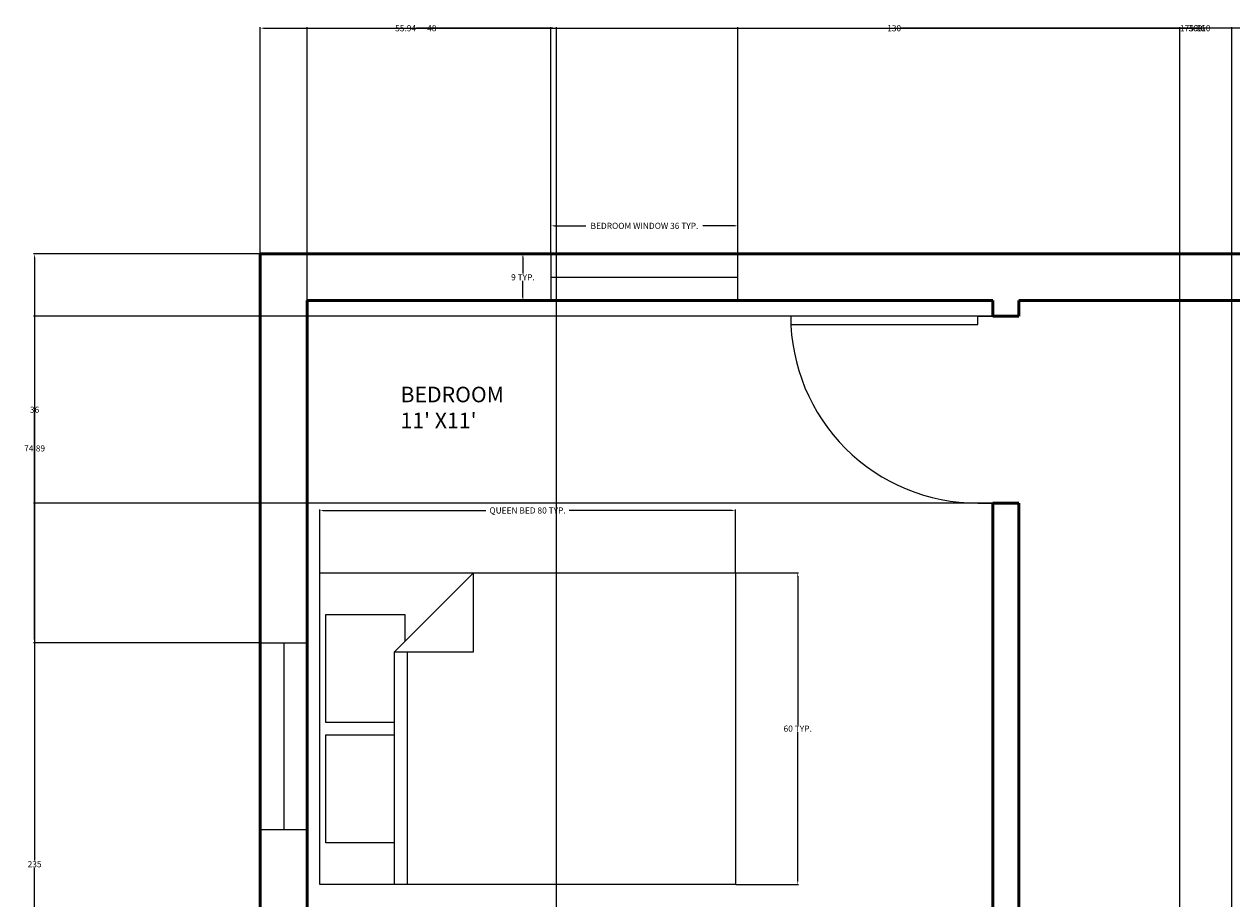
# Model space of a CAD drawing. Units: inches. Extents: x 3506 to 3958, y 1553 to 2506.
# Tile 14 of 16: x 3506 to 3739, y 2337 to 2506. Entities that reach past the tile are written whole.
import ezdxf

# ---------------------------------------------------------------- set-up
doc = ezdxf.new("R2010")
doc.units = ezdxf.units.IN
doc.header["$MEASUREMENT"] = 0
for name, color, linetype, lineweight in [('A-ANNO-DIMS', 2, 'Continuous', 18), ('A-AREA-IDEN', 7, 'Continuous', 18), ('A-WALL', 7, 'Continuous', 50), ('doors', 40, 'Continuous', 25), ('furniture', 120, 'Continuous', 18), ('window', 30, 'Continuous', 20)]:
    doc.layers.add(name, color=color, linetype=linetype, lineweight=lineweight)
doc.layers.add('A-WALL-PATT', color=251, linetype='Continuous', lineweight=13, true_color=0x636466)
doc.styles.get("Standard").update_dxf_attribs({"font": 'arial.ttf'})
doc.dimstyles.get("Standard").update_dxf_attribs({"dimtxt": 1.18, "dimasz": 0.68, "dimexe": 0.18, "dimexo": 0.0625, "dimgap": 0.09, "dimtad": 0, "dimtih": 1, "dimtoh": 1, "dimdec": 1, "dimzin": 0, "dimdsep": 46, "dimlunit": 3, "dimtxsty": 'Standard', "dimcen": 0.09, "dimadec": 0, "dimazin": 0, "dimtfac": 1, "dimtdec": 1, "dimtofl": 0, "dimtmove": 0, "dimatfit": 3, "dimfxl": 1, "dimtolj": 1, "dimtzin": 0, "dimarcsym": 0})

# ---------------------------------------------------------------- blocks, each defined once
blk = doc.blocks.new('*U12')
for p, q in [((0, 0), (0, 6)), ((40, 0), (40, 6))]:
    blk.add_line(p, q)
blk.add_lwpolyline([(0, 0), (0, -40), (1.75, -40), (1.75, 0)], close=True)
blk.add_arc((0, 0), 40, 270, 0)
blk = doc.blocks.new('Bed - Queen')
for p, q in [((0, -80.00003), (0, 0)), ((0, 0), (59.99999, 0)), ((59.99999, 0), (59.99999, -80.00003)), ((7.99999, -1.2), (28.79998, -1.2)), ((7.99999, -14.4), (7.99999, -1.2)), ((28.79998, -1.2), (28.79998, -14.4)), ((31.19999, -1.2), (51.99999, -1.2)), ((31.19999, -14.4), (31.19999, -1.2)), ((51.99999, -1.2), (51.99999, -16.4)), ((0, -14.4), (44.8, -14.4)), ((59.99999, -29.6), (44.8, -14.4)), ((44.8, -14.4), (44.8, -29.6)), ((44.8, -16.8), (0, -16.8)), ((51.99999, -16.4), (46.79936, -16.4)), ((44.8, -29.6), (59.99999, -29.6)), ((59.99999, -80.00003), (0, -80.00003))]:
    blk.add_line(p, q)
blk = doc.blocks.new('WIN-36IN-9IN-WALL')
for p, q in [((0, 9), (0, 0)), ((36, 9), (0, 9)), ((0, 9), (0, 4.5)), ((36, 0), (36, 9)), ((0, 4.5), (36, 4.5)), ((0, 0), (36, 0))]:
    blk.add_line(p, q)
blk = doc.blocks.new('*D18')
at = {"layer": 'A-ANNO-DIMS', "color": 0, "lineweight": -2, "transparency": 16777216}
for p, q in [((3563.17, 2400.06), (3563.17, 2412.18)), ((3563.85, 2412), (3595.12, 2412)), ((3642.49, 2412), (3611.21, 2412)), ((3643.17, 2400.06), (3643.17, 2412.18))]:
    blk.add_line(p, q, dxfattribs=at)
at = {"layer": 'A-ANNO-DIMS', "color": 0, "transparency": 16777216}
for points in [[(3563.85, 2412.11), (3563.85, 2411.89), (3563.17, 2412)], [(3642.49, 2412.11), (3642.49, 2411.89), (3643.17, 2412)]]:
    blk.add_solid(points, dxfattribs=at)
at = {"layer": 'Defpoints', "color": 0, "transparency": 16777216}
for p in [(3563.17, 2412), (3563.17, 2400), (3643.17, 2400)]:
    blk.add_point(p, dxfattribs=at)
at = {"layer": 'A-ANNO-DIMS', "color": 0, "transparency": 16777216, "insert": (3603.17, 2412), "char_height": 1.18, "attachment_point": 5}
blk.add_mtext('\\A1;QUEEN BED 80 TYP.', dxfattribs=at)
blk = doc.blocks.new('*D19')
at = {"layer": 'A-ANNO-DIMS', "color": 0, "lineweight": -2, "transparency": 16777216}
for p, q in [((3643.23, 2400), (3655.35, 2400)), ((3655.17, 2399.32), (3655.17, 2370.69)), ((3655.17, 2340.68), (3655.17, 2369.31)), ((3643.23, 2340), (3655.35, 2340))]:
    blk.add_line(p, q, dxfattribs=at)
at = {"layer": 'A-ANNO-DIMS', "color": 0, "transparency": 16777216}
for points in [[(3655.06, 2399.32), (3655.28, 2399.32), (3655.17, 2400)], [(3655.06, 2340.68), (3655.28, 2340.68), (3655.17, 2340)]]:
    blk.add_solid(points, dxfattribs=at)
at = {"layer": 'Defpoints', "color": 0, "transparency": 16777216}
for p in [(3643.17, 2400), (3655.17, 2400), (3643.17, 2340)]:
    blk.add_point(p, dxfattribs=at)
at = {"layer": 'A-ANNO-DIMS', "color": 0, "transparency": 16777216, "insert": (3655.17, 2370), "char_height": 1.18, "attachment_point": 5}
blk.add_mtext('\\A1;60 TYP.', dxfattribs=at)
blk = doc.blocks.new('*D32')
at = {"layer": 'A-ANNO-DIMS', "color": 0, "lineweight": -2, "transparency": 16777216}
for p, q in [((3607.67, 2461.46), (3607.67, 2466.97)), ((3608.35, 2466.79), (3614.4, 2466.79)), ((3642.99, 2466.79), (3636.94, 2466.79)), ((3643.67, 2461.46), (3643.67, 2466.97))]:
    blk.add_line(p, q, dxfattribs=at)
at = {"layer": 'A-ANNO-DIMS', "color": 0, "transparency": 16777216}
for points in [[(3608.35, 2466.91), (3608.35, 2466.68), (3607.67, 2466.79)], [(3642.99, 2466.91), (3642.99, 2466.68), (3643.67, 2466.79)]]:
    blk.add_solid(points, dxfattribs=at)
at = {"layer": 'Defpoints', "color": 0, "transparency": 16777216}
for p in [(3643.67, 2466.79), (3607.67, 2461.39), (3643.67, 2461.39)]:
    blk.add_point(p, dxfattribs=at)
at = {"layer": 'A-ANNO-DIMS', "color": 0, "transparency": 16777216, "insert": (3625.67, 2466.79), "char_height": 1.18, "attachment_point": 5}
blk.add_mtext('\\A1;BEDROOM WINDOW 36 TYP.', dxfattribs=at)
blk = doc.blocks.new('*D33')
at = {"layer": 'A-ANNO-DIMS', "color": 0, "lineweight": -2, "transparency": 16777216}
for p, q in [((3607.6, 2461.39), (3602.09, 2461.39)), ((3602.27, 2460.71), (3602.27, 2457.59)), ((3602.27, 2453.07), (3602.27, 2456.2)), ((3607.6, 2452.39), (3602.09, 2452.39))]:
    blk.add_line(p, q, dxfattribs=at)
at = {"layer": 'A-ANNO-DIMS', "color": 0, "transparency": 16777216}
for points in [[(3602.15, 2460.71), (3602.38, 2460.71), (3602.27, 2461.39)], [(3602.15, 2453.07), (3602.38, 2453.07), (3602.27, 2452.39)]]:
    blk.add_solid(points, dxfattribs=at)
at = {"layer": 'Defpoints', "color": 0, "transparency": 16777216}
for p in [(3602.27, 2461.39), (3607.67, 2461.39), (3607.67, 2452.39)]:
    blk.add_point(p, dxfattribs=at)
at = {"layer": 'A-ANNO-DIMS', "color": 0, "transparency": 16777216, "insert": (3602.27, 2456.89), "char_height": 1.18, "attachment_point": 5}
blk.add_mtext('\\A1;9 TYP.', dxfattribs=at)
blk = doc.blocks.new('*D38')
at = {"layer": 'A-ANNO-DIMS', "color": 0, "lineweight": -2, "transparency": 16777216}
for p, q in [((3551.73, 2461.46), (3551.73, 2505.02)), ((3552.41, 2504.84), (3730.34, 2504.84)), ((3911.05, 2504.84), (3733.12, 2504.84)), ((3911.73, 2461.46), (3911.73, 2505.02))]:
    blk.add_line(p, q, dxfattribs=at)
at = {"layer": 'A-ANNO-DIMS', "color": 0, "transparency": 16777216}
for points in [[(3552.41, 2504.96), (3552.41, 2504.73), (3551.73, 2504.84)], [(3911.05, 2504.96), (3911.05, 2504.73), (3911.73, 2504.84)]]:
    blk.add_solid(points, dxfattribs=at)
at = {"layer": 'Defpoints', "color": 0, "transparency": 16777216}
for p in [(3911.73, 2504.84), (3551.73, 2461.39), (3911.73, 2461.39)]:
    blk.add_point(p, dxfattribs=at)
at = {"layer": 'A-ANNO-DIMS', "color": 0, "transparency": 16777216, "insert": (3731.73, 2504.84), "char_height": 1.18, "attachment_point": 5}
blk.add_mtext('\\A1;360', dxfattribs=at)
blk = doc.blocks.new('*D44')
at = {"layer": 'A-ANNO-DIMS', "color": 0, "lineweight": -2, "transparency": 16777216}
for p, q in [((3911.67, 2461.39), (3508.1, 2461.39)), ((3508.28, 2460.71), (3508.28, 2344.59)), ((3508.28, 2227.07), (3508.28, 2343.2)), ((3560.67, 2226.39), (3508.1, 2226.39))]:
    blk.add_line(p, q, dxfattribs=at)
at = {"layer": 'A-ANNO-DIMS', "color": 0, "transparency": 16777216}
for points in [[(3508.17, 2460.71), (3508.39, 2460.71), (3508.28, 2461.39)], [(3508.17, 2227.07), (3508.39, 2227.07), (3508.28, 2226.39)]]:
    blk.add_solid(points, dxfattribs=at)
at = {"layer": 'Defpoints', "color": 0, "transparency": 16777216}
for p in [(3508.28, 2461.39), (3911.73, 2461.39), (3560.73, 2226.39)]:
    blk.add_point(p, dxfattribs=at)
at = {"layer": 'A-ANNO-DIMS', "color": 0, "transparency": 16777216, "insert": (3508.28, 2343.89), "char_height": 1.18, "attachment_point": 5}
blk.add_mtext('\\A1;235', dxfattribs=at)
blk = doc.blocks.new('*D45')
at = {"layer": 'A-ANNO-DIMS', "color": 0, "lineweight": -2, "transparency": 16777216}
for p, q in [((3551.73, 2461.46), (3551.73, 2505.02)), ((3552.41, 2504.84), (3577.62, 2504.84)), ((3606.99, 2504.84), (3581.78, 2504.84)), ((3607.67, 2461.46), (3607.67, 2505.02))]:
    blk.add_line(p, q, dxfattribs=at)
at = {"layer": 'A-ANNO-DIMS', "color": 0, "transparency": 16777216}
for points in [[(3552.41, 2504.96), (3552.41, 2504.73), (3551.73, 2504.84)], [(3606.99, 2504.96), (3606.99, 2504.73), (3607.67, 2504.84)]]:
    blk.add_solid(points, dxfattribs=at)
at = {"layer": 'Defpoints', "color": 0, "transparency": 16777216}
for p in [(3607.67, 2504.84), (3551.73, 2461.39), (3607.67, 2461.39)]:
    blk.add_point(p, dxfattribs=at)
at = {"layer": 'A-ANNO-DIMS', "color": 0, "transparency": 16777216, "insert": (3579.7, 2504.84), "char_height": 1.18, "attachment_point": 5}
blk.add_mtext('\\A1;55.94', dxfattribs=at)
blk = doc.blocks.new('*D46')
at = {"layer": 'A-ANNO-DIMS', "color": 0, "lineweight": -2, "transparency": 16777216}
for p, q in [((3643.67, 2461.46), (3643.67, 2505.02)), ((3644.35, 2504.84), (3728.72, 2504.84)), ((3818.05, 2504.84), (3733.68, 2504.84)), ((3818.73, 2461.46), (3818.73, 2505.02))]:
    blk.add_line(p, q, dxfattribs=at)
at = {"layer": 'A-ANNO-DIMS', "color": 0, "transparency": 16777216}
for points in [[(3644.35, 2504.96), (3644.35, 2504.73), (3643.67, 2504.84)], [(3818.05, 2504.96), (3818.05, 2504.73), (3818.73, 2504.84)]]:
    blk.add_solid(points, dxfattribs=at)
at = {"layer": 'Defpoints', "color": 0, "transparency": 16777216}
for p in [(3818.73, 2504.84), (3643.67, 2461.39), (3818.73, 2461.39)]:
    blk.add_point(p, dxfattribs=at)
at = {"layer": 'A-ANNO-DIMS', "color": 0, "transparency": 16777216, "insert": (3731.2, 2504.84), "char_height": 1.18, "attachment_point": 5}
blk.add_mtext('\\A1;175.06', dxfattribs=at)
blk = doc.blocks.new('*D50')
at = {"layer": 'A-ANNO-DIMS', "color": 0, "lineweight": -2, "transparency": 16777216}
for p, q in [((3608.73, 1606.46), (3608.73, 2505.02)), ((3609.41, 2504.84), (3672.39, 2504.84)), ((3738.05, 2504.84), (3675.07, 2504.84)), ((3738.73, 1606.46), (3738.73, 2505.02))]:
    blk.add_line(p, q, dxfattribs=at)
at = {"layer": 'A-ANNO-DIMS', "color": 0, "transparency": 16777216}
for points in [[(3609.41, 2504.96), (3609.41, 2504.73), (3608.73, 2504.84)], [(3738.05, 2504.96), (3738.05, 2504.73), (3738.73, 2504.84)]]:
    blk.add_solid(points, dxfattribs=at)
at = {"layer": 'Defpoints', "color": 0, "transparency": 16777216}
for p in [(3738.73, 2504.84), (3608.73, 1606.39), (3738.73, 1606.39)]:
    blk.add_point(p, dxfattribs=at)
at = {"layer": 'A-ANNO-DIMS', "color": 0, "transparency": 16777216, "insert": (3673.73, 2504.84), "char_height": 1.18, "attachment_point": 5}
blk.add_mtext('\\A1;130', dxfattribs=at)
blk = doc.blocks.new('*D52')
at = {"layer": 'A-ANNO-DIMS', "color": 0, "lineweight": -2, "transparency": 16777216}
for p, q in [((3560.73, 1606.46), (3560.73, 2505.02)), ((3561.41, 2504.84), (3583.77, 2504.84)), ((3608.05, 2504.84), (3585.69, 2504.84)), ((3608.73, 1606.46), (3608.73, 2505.02))]:
    blk.add_line(p, q, dxfattribs=at)
at = {"layer": 'A-ANNO-DIMS', "color": 0, "transparency": 16777216}
for points in [[(3561.41, 2504.96), (3561.41, 2504.73), (3560.73, 2504.84)], [(3608.05, 2504.96), (3608.05, 2504.73), (3608.73, 2504.84)]]:
    blk.add_solid(points, dxfattribs=at)
at = {"layer": 'Defpoints', "color": 0, "transparency": 16777216}
for p in [(3608.73, 2504.84), (3560.73, 1606.39), (3608.73, 1606.39)]:
    blk.add_point(p, dxfattribs=at)
at = {"layer": 'A-ANNO-DIMS', "color": 0, "transparency": 16777216, "insert": (3584.73, 2504.84), "char_height": 1.18, "attachment_point": 5}
blk.add_mtext('\\A1;48', dxfattribs=at)
blk = doc.blocks.new('*D55')
at = {"layer": 'A-ANNO-DIMS', "color": 0, "lineweight": -2, "transparency": 16777216}
for p, q in [((3551.67, 2461.39), (3508.1, 2461.39)), ((3508.28, 2460.71), (3508.28, 2424.64)), ((3508.28, 2387.19), (3508.28, 2423.26)), ((3551.67, 2386.51), (3508.1, 2386.51))]:
    blk.add_line(p, q, dxfattribs=at)
at = {"layer": 'A-ANNO-DIMS', "color": 0, "transparency": 16777216}
for points in [[(3508.17, 2460.71), (3508.39, 2460.71), (3508.28, 2461.39)], [(3508.17, 2387.19), (3508.39, 2387.19), (3508.28, 2386.51)]]:
    blk.add_solid(points, dxfattribs=at)
at = {"layer": 'Defpoints', "color": 0, "transparency": 16777216}
for p in [(3551.73, 2461.39), (3508.28, 2386.51), (3551.73, 2386.51)]:
    blk.add_point(p, dxfattribs=at)
at = {"layer": 'A-ANNO-DIMS', "color": 0, "transparency": 16777216, "insert": (3508.28, 2423.95), "char_height": 1.18, "attachment_point": 5}
blk.add_mtext('\\A1;74.89', dxfattribs=at)
blk = doc.blocks.new('*D56')
at = {"layer": 'A-ANNO-DIMS', "color": 0, "lineweight": -2, "transparency": 16777216}
for p, q in [((3692.67, 2449.39), (3508.1, 2449.39)), ((3508.28, 2448.71), (3508.28, 2432.09)), ((3508.28, 2414.07), (3508.28, 2430.7)), ((3692.67, 2413.39), (3508.1, 2413.39))]:
    blk.add_line(p, q, dxfattribs=at)
at = {"layer": 'A-ANNO-DIMS', "color": 0, "transparency": 16777216}
for points in [[(3508.17, 2448.71), (3508.39, 2448.71), (3508.28, 2449.39)], [(3508.17, 2414.07), (3508.39, 2414.07), (3508.28, 2413.39)]]:
    blk.add_solid(points, dxfattribs=at)
at = {"layer": 'Defpoints', "color": 0, "transparency": 16777216}
for p in [(3692.73, 2449.39), (3508.28, 2413.39), (3692.73, 2413.39)]:
    blk.add_point(p, dxfattribs=at)
at = {"layer": 'A-ANNO-DIMS', "color": 0, "transparency": 16777216, "insert": (3508.28, 2431.39), "char_height": 1.18, "attachment_point": 5}
blk.add_mtext('\\A1;36', dxfattribs=at)
blk = doc.blocks.new('*D59')
at = {"layer": 'A-ANNO-DIMS', "color": 0, "lineweight": -2, "transparency": 16777216}
for p, q in [((3728.73, 1689.46), (3728.73, 2505.02)), ((3729.41, 2504.84), (3732.85, 2504.84)), ((3738.05, 2504.84), (3734.61, 2504.84)), ((3738.73, 1689.46), (3738.73, 2505.02))]:
    blk.add_line(p, q, dxfattribs=at)
at = {"layer": 'A-ANNO-DIMS', "color": 0, "transparency": 16777216}
for points in [[(3729.41, 2504.96), (3729.41, 2504.73), (3728.73, 2504.84)], [(3738.05, 2504.96), (3738.05, 2504.73), (3738.73, 2504.84)]]:
    blk.add_solid(points, dxfattribs=at)
at = {"layer": 'Defpoints', "color": 0, "transparency": 16777216}
for p in [(3738.73, 2504.84), (3728.73, 1689.39), (3738.73, 1689.39)]:
    blk.add_point(p, dxfattribs=at)
at = {"layer": 'A-ANNO-DIMS', "color": 0, "transparency": 16777216, "insert": (3733.73, 2504.84), "char_height": 1.18, "attachment_point": 5}
blk.add_mtext('\\A1;10', dxfattribs=at)

msp = doc.modelspace()

# ---------------------------------------------------------------- hatches: boundary and pattern name
at = {"layer": 'A-WALL-PATT'}
h = msp.add_hatch(dxfattribs=at)
h.set_pattern_fill('ANSI31', color=256)
h.paths.add_polyline_path([(3911.7302, 2461.3942), (3551.7302, 2461.3942), (3551.7302, 2152.516), (3560.7302, 2152.516), (3560.7302, 2116.516), (3551.7302, 2116.516), (3551.7302, 1920.5711), (3556.2302, 1920.5711), (3560.7302, 1920.5711), (3560.7302, 2000.3942), (3692.7302, 2000.3942), (3692.7302, 1997.3942), (3697.7302, 1997.3942), (3697.7302, 2000.3942), (3771.7302, 2000.3942), (3771.7302, 1997.3942), (3776.7302, 1997.3942), (3776.7302, 1997.7206), (3778.5802, 1997.7206), (3807.5802, 1997.7206), (3807.5802, 1996.4519), (3778.5802, 1996.4519), (3778.5802, 1997.7206), (3776.7302, 1997.7206), (3776.7302, 1997.3942), (3771.7302, 1997.3942), (3771.7302, 2000.3942), (3697.7302, 2000.3942), (3697.7302, 1997.3942), (3692.7302, 1997.3942), (3689.8302, 1997.3942), (3689.8302, 1995.8192), (3653.8302, 1995.8192), (3653.8302, 1997.3942), (3689.8302, 1997.3942), (3692.7302, 1997.3942), (3692.7302, 2000.3942), (3560.7302, 2000.3942), (3560.7302, 1920.5711), (3551.7302, 1920.5711), (3551.7302, 1884.5711), (3551.7302, 1597.3942), (3911.7302, 1597.3942)], flags=17)
h.paths.add_polyline_path([(3596.7302, 2005.3942), (3596.7302, 2057.3035, -0.38730371), (3569.1778, 2085), (3569.15, 2085), (3569.15, 2086.2688), (3598.15, 2086.2688), (3598.15, 2085), (3569.1778, 2085, 0.38730371), (3596.7302, 2057.3035), (3596.7302, 2057.3942), (3601.7302, 2057.3942), (3601.7302, 2055.3942), (3630.7302, 2055.3942), (3630.7302, 2034.3942), (3694.7302, 2034.3942), (3694.7302, 2053.3942), (3699.7302, 2053.3942), (3699.7302, 2005.3942), (3860.7302, 2005.3942), (3860.7302, 2173.3942), (3771.7302, 2173.3942), (3771.7302, 2194.3942), (3776.7302, 2194.3942), (3776.7302, 2178.3942), (3860.7302, 2178.3942), (3860.7302, 2231.3942), (3601.7302, 2231.3942), (3601.7302, 2241.426), (3596.7302, 2241.426), (3596.7302, 2231.3942), (3560.7302, 2231.3942), (3560.7302, 2315.3942), (3596.7302, 2315.3942), (3596.7302, 2312.3942), (3601.7302, 2312.3942), (3601.7302, 2315.3942), (3697.7302, 2315.3942), (3697.7302, 2413.3942), (3692.7302, 2413.3942), (3692.7302, 2320.3942), (3560.7302, 2320.3942), (3560.7302, 2452.3942), (3692.7302, 2452.3942), (3692.7302, 2449.3942), (3697.7302, 2449.3942), (3697.7302, 2452.3942), (3771.7302, 2452.3942), (3771.7302, 2449.3942), (3776.7302, 2449.3942), (3776.7302, 2452.3942), (3860.7302, 2452.3942), (3860.7302, 2437.2075), (3865.2302, 2437.2075), (3865.2302, 2413.2075), (3860.7302, 2413.2075), (3860.7302, 2367.6976), (3865.2302, 2367.6976), (3869.7302, 2367.6976), (3869.7302, 2319.6976), (3860.7302, 2319.6976), (3860.7302, 2211.6248), (3869.7302, 2211.6248), (3869.7302, 2187.6248), (3860.7302, 2187.6248), (3860.7302, 2138.4346), (3865.2302, 2138.4346), (3869.7302, 2138.4346), (3869.7302, 2090.4346), (3860.7302, 2090.4346), (3860.7302, 1985.8449), (3869.7302, 1985.8449), (3869.7302, 1961.8449), (3860.7302, 1961.8449), (3860.7302, 1897.0756), (3865.2302, 1897.0756), (3869.7302, 1897.0756), (3869.7302, 1849.0756), (3860.7302, 1849.0756), (3860.7302, 1847.8112), (3860.7302, 1779.3942), (3596.7302, 1779.3942), (3596.7302, 1831.3942), (3601.7302, 1831.3942), (3601.7302, 1828.3942), (3630.7302, 1828.3942), (3630.7302, 1808.3942), (3691.7302, 1808.3942), (3691.7302, 1815.3942), (3696.7302, 1815.3942), (3696.7302, 1779.3942), (3860.7302, 1779.3942), (3860.7302, 1947.3942), (3771.7302, 1947.3942), (3771.7302, 1968.3942), (3776.7302, 1968.3942), (3776.7302, 1952.3942), (3860.7302, 1952.3942), (3860.7302, 2005.3942)], flags=0)
h.paths.add_polyline_path([(3596.7302, 2038.8546), (3601.7302, 2038.8546), (3601.7302, 2014.8546), (3596.7302, 2014.8546)], flags=0)
h.paths.add_polyline_path([(3564.1688, 2107), (3564.1688, 2167), (3644.1688, 2167), (3644.1688, 2107)], flags=0)
h.paths.add_polyline_path([(3607.0972, 2052.0208), (3620.8472, 2052.0208, -0.41421356), (3621.9931, 2050.875), (3621.9931, 2025.6667, -0.41421356), (3620.8472, 2024.5208), (3607.0972, 2024.5208, -0.41421356), (3605.9514, 2025.6667), (3605.9514, 2050.875, -0.41421356)], flags=0)
h.paths.add_polyline_path([(3578.5688, 2115), (3565.3688, 2115), (3565.3688, 2135.8), (3578.5688, 2135.8), (3578.5688, 2138.2), (3565.3688, 2138.2), (3565.3688, 2159), (3580.5688, 2159), (3580.5688, 2153.8), (3593.7688, 2167), (3593.7688, 2151.8), (3578.5688, 2151.8)], flags=0)
h.paths.add_polyline_path([(3610.9167, 2050.875), (3620.0833, 2050.875, -0.41421356), (3620.8472, 2050.1111), (3620.8472, 2039.6076, -0.41421356), (3620.0833, 2038.8438), (3610.9167, 2038.8438, -0.41421356), (3610.1528, 2039.6076), (3610.1528, 2050.1111, -0.41421356)], flags=0)
h.paths.add_polyline_path([(3610.9167, 2037.6979), (3620.0833, 2037.6979, -0.41421356), (3620.8472, 2036.934), (3620.8472, 2026.4306, -0.41421356), (3620.0833, 2025.6667), (3610.9167, 2025.6667, -0.41421356), (3610.1528, 2026.4306), (3610.1528, 2036.934, -0.41421356)], flags=0)
h.paths.add_polyline_path([(3616.2639, 2044.7639, -1), (3614.7361, 2044.7639, -1)], flags=0)
h.paths.add_polyline_path([(3615.8819, 2044.7639, -1), (3615.1181, 2044.7639, -1)], flags=0)
h.paths.add_polyline_path([(3616.2639, 2031.7778, -1), (3614.7361, 2031.7778, -1)], flags=0)
h.paths.add_polyline_path([(3615.8819, 2031.7778, -1), (3615.1181, 2031.7778, -1)], flags=0)
h.paths.add_polyline_path([(3609.7539, 2021.7868), (3626.9586, 2021.7868), (3626.9586, 2008.8833), (3609.7539, 2008.8833)], flags=0)
h.paths.add_polyline_path([(3610.4708, 2021.07), (3621.2237, 2021.07), (3621.2237, 2009.6002), (3610.4708, 2009.6002)], flags=0)
h.paths.add_polyline_path([(3611.5461, 2019.9947), (3620.1484, 2019.9947), (3620.1484, 2010.6755), (3611.5461, 2010.6755)], flags=0)
h.paths.add_polyline_path([(3621.9405, 2021.07), (3626.2417, 2021.07), (3626.2417, 2009.6002), (3621.9405, 2009.6002)], flags=0)
h.paths.add_polyline_path([(3622.6574, 2020.3531), (3625.5248, 2020.3531), (3625.5248, 2017.4857), (3622.6574, 2017.4857)], flags=0)
h.paths.add_polyline_path([(3622.6574, 2016.7688), (3625.5248, 2016.7688), (3625.5248, 2010.317), (3622.6574, 2010.317)], flags=0)
h.paths.add_polyline_path([(3624.808, 2016.0519), (3624.808, 2013.9013), (3624.0911, 2013.9013), (3624.0911, 2013.1845), (3623.3743, 2013.1845), (3623.3743, 2013.9013), (3623.3743, 2016.0519)], flags=0)
h.paths.add_polyline_path([(3623.0158, 2012.8261), (3625.1664, 2012.8261), (3625.1664, 2012.1092), (3623.0158, 2012.1092)], flags=0)
h.paths.add_polyline_path([(3623.0158, 2011.7508), (3625.1664, 2011.7508), (3625.1664, 2011.0339), (3623.0158, 2011.0339)], flags=0)
h.paths.add_polyline_path([(3650.0591, 2031.8202), (3674.0368, 2031.8202), (3674.0368, 2012.638), (3669.2413, 2012.638), (3669.2413, 2011.8388), (3672.4383, 2011.8388), (3672.4383, 2011.0395), (3651.6576, 2011.0395), (3651.6576, 2011.8388), (3654.8546, 2011.8388), (3654.8546, 2012.638), (3650.0591, 2012.638)], flags=0)
h.paths.add_polyline_path([(3658.0517, 2024.6269, -1), (3651.6576, 2024.6269, -1)], flags=0)
h.paths.add_polyline_path([(3657.2524, 2024.6269, -1), (3652.4569, 2024.6269, -1)], flags=0)
h.paths.add_polyline_path([(3656.4532, 2024.6269, -1), (3653.2561, 2024.6269, -1)], flags=0)
h.paths.add_polyline_path([(3655.6539, 2024.6269, -1), (3654.0554, 2024.6269, -1)], flags=0)
h.paths.add_polyline_path([(3657.2524, 2017.4336, -1), (3652.4569, 2017.4336, -1)], flags=0)
h.paths.add_polyline_path([(3656.4532, 2017.4336, -1), (3653.2561, 2017.4336, -1)], flags=0)
h.paths.add_polyline_path([(3655.6539, 2017.4336, -1), (3654.0554, 2017.4336, -1)], flags=0)
h.paths.add_polyline_path([(3659.6502, 2027.8239), (3664.4457, 2027.8239), (3664.4457, 2015.0358), (3659.6502, 2015.0358)], flags=0)
h.paths.add_polyline_path([(3663.6465, 2027.0247), (3663.6465, 2015.8351), (3660.4494, 2015.8351), (3660.4494, 2027.0247)], flags=0)
h.paths.add_polyline_path([(3562.6688, 1945.5), (3642.6688, 1945.5), (3642.6688, 1885.5), (3562.6688, 1885.5)], flags=0)
h.paths.add_polyline_path([(3671.6391, 2024.6269, -1), (3666.8435, 2024.6269, -1)], flags=0)
h.paths.add_polyline_path([(3670.8398, 2024.6269, -1), (3667.6428, 2024.6269, -1)], flags=0)
h.paths.add_polyline_path([(3672.4383, 2017.4336, -1), (3666.0443, 2017.4336, -1)], flags=0)
h.paths.add_polyline_path([(3670.0405, 2024.6269, -1), (3668.442, 2024.6269, -1)], flags=0)
h.paths.add_polyline_path([(3671.6391, 2017.4336, -1), (3666.8435, 2017.4336, -1)], flags=0)
h.paths.add_polyline_path([(3670.8398, 2017.4336, -1), (3667.6428, 2017.4336, -1)], flags=0)
h.paths.add_polyline_path([(3592.2688, 1945.5), (3592.2688, 1930.3), (3577.0688, 1930.3), (3577.0688, 1893.5), (3563.8688, 1893.5), (3563.8688, 1914.3), (3577.0688, 1914.3), (3577.0688, 1916.7), (3563.8688, 1916.7), (3563.8688, 1937.5), (3579.0688, 1937.5), (3579.0688, 1932.3)], flags=0)
h.paths.add_polyline_path([(3670.0405, 2017.4336, -1), (3668.442, 2017.4336, -1)], flags=0)
h.paths.add_polyline_path([(3596.7302, 2283.3942), (3601.7302, 2283.3942), (3601.7302, 2265.426), (3599.2302, 2265.426), (3599.2302, 2241.426), (3596.7302, 2241.426), (3596.7302, 2265.426)], flags=0)
h.paths.add_polyline_path([(3596.7302, 1810.7006), (3601.7302, 1810.7006), (3601.7302, 1786.7006), (3596.7302, 1786.7006)], flags=0)
h.paths.add_polyline_path([(3560.7302, 1770.3942), (3738.7302, 1770.3942), (3738.7302, 1746.3942), (3738.7302, 1722.3942), (3748.7302, 1722.3942), (3748.7302, 1674.3942), (3560.7302, 1674.3942)], flags=0)
h.paths.add_polyline_path([(3728.7302, 1746.3942), (3728.7302, 1756.0642), (3738.7302, 1746.3942), (3728.7302, 1738.1582), (3728.7302, 1698.3942), (3591.2519, 1698.3942), (3591.2519, 1746.3942)], flags=0)
h.paths.add_polyline_path([(3771.7302, 2399.3942), (3771.7302, 2420.3942), (3776.7302, 2420.3942), (3776.7302, 2404.3942), (3776.7302, 2399.3942)], flags=0)
h.paths.add_polyline_path([(3911.7302, 2461.3942), (3551.7302, 2461.3942), (3551.7302, 2152.516), (3560.7302, 2152.516), (3560.7302, 2116.516), (3551.7302, 2116.516), (3551.7302, 1920.5711), (3560.7302, 1920.5711), (3560.7302, 2000.3942), (3692.7302, 2000.3942), (3692.7302, 1997.3942), (3697.7302, 1997.3942), (3697.7302, 2000.3942), (3771.7302, 2000.3942), (3771.7302, 1997.3942), (3776.7302, 1997.3942), (3776.7302, 1997.7206), (3778.5802, 1997.7206), (3807.5802, 1997.7206), (3807.5802, 1996.4519), (3778.5802, 1996.4519), (3778.5802, 1997.7206), (3776.7302, 1997.7206), (3776.7302, 1997.3942), (3771.7302, 1997.3942), (3771.7302, 2000.3942), (3697.7302, 2000.3942), (3697.7302, 1997.3942), (3692.7302, 1997.3942), (3689.8302, 1997.3942), (3689.8302, 1995.8192), (3653.8302, 1995.8192), (3653.8302, 1997.3942), (3689.8302, 1997.3942), (3692.7302, 1997.3942), (3692.7302, 2000.3942), (3560.7302, 2000.3942), (3560.7302, 1920.5711), (3551.7302, 1920.5711), (3551.7302, 1597.3942), (3911.7302, 1597.3942)], flags=17)

# ---------------------------------------------------------------- linework, layer by layer
at = {"layer": 'A-WALL'}
for p, q in [((3560.7302, 2452.3942), (3692.7302, 2452.3942)), ((3560.7302, 2320.3942), (3560.7302, 2452.3942)), ((3692.7302, 2452.3942), (3692.7302, 2449.3942)), ((3692.7302, 2449.3942), (3692.7302, 2452.3942)), ((3692.7302, 2449.3942), (3692.7302, 2452.3942)), ((3697.7302, 2452.3942), (3771.7302, 2452.3942)), ((3697.7302, 2449.3942), (3697.7302, 2452.3942)), ((3697.7302, 2449.3942), (3697.7302, 2452.3942)), ((3692.7302, 2449.3942), (3697.7302, 2449.3942)), ((3692.7302, 2320.3942), (3692.7302, 2413.3942)), ((3692.7302, 2320.3942), (3692.7302, 2413.3942)), ((3692.7302, 2413.3942), (3697.7302, 2413.3942)), ((3697.7302, 2320.3942), (3697.7302, 2413.3942)), ((3697.7302, 2315.3942), (3697.7302, 2413.3942))]:
    msp.add_line(p, q, dxfattribs=at)
msp.add_lwpolyline([(3551.7302, 2461.3942), (3911.7302, 2461.3942), (3911.7302, 1597.3942), (3551.7302, 1597.3942)], close=True, dxfattribs=at)

# ---------------------------------------------------------------- block references
at = {"layer": 'doors', "xscale": 0.9000000000000001, "yscale": 0.9000000000000001, "zscale": 0.9000000000000001, "rotation": 270}
msp.add_blockref('*U12', (3689.8302, 2449.3942), dxfattribs=at)
at = {"layer": 'furniture', "rotation": 90}
msp.add_blockref('Bed - Queen', (3563.1688, 2340), dxfattribs=at)
at = {"layer": 'window'}
msp.add_blockref('WIN-36IN-9IN-WALL', (3607.667, 2452.394), dxfattribs=at)
at = {"layer": 'window', "extrusion": (0, 0, -1), "zscale": -1, "rotation": 269.9999999999985}
msp.add_blockref('WIN-36IN-9IN-WALL', (-3560.7304, 2386.5074), dxfattribs=at)

# ---------------------------------------------------------------- texts
at = {"layer": 'A-AREA-IDEN', "insert": (3578.7164, 2435.824), "char_height": 3, "attachment_point": 1}
msp.add_mtext_dynamic_manual_height_columns("BEDROOM\\P11' X11'", width=46.119714, gutter_width=1, heights=[0], dxfattribs=at)

# ---------------------------------------------------------------- dimensions: what is measured, and where the dimension line sits
at = {"layer": 'A-ANNO-DIMS'}
for base, p1, p2, override, picture, middle in [((3911.7302, 2504.8442), (3551.7302, 2461.3942), (3911.7302, 2461.3942), {"dimdec": 0, "dimlfac": 1, "dimrnd": 0, "dimzin": 0, "dimdsep": 46, "dimlunit": 2}, '*D38', (3731.7302, 2504.8442)), ((3607.667, 2504.8442), (3551.7302, 2461.3942), (3607.667, 2461.3942), {"dimdec": 2, "dimlfac": 1, "dimrnd": 0, "dimzin": 0, "dimdsep": 46, "dimlunit": 2}, '*D45', (3579.6986, 2504.8442)), ((3608.7302, 2504.8442), (3560.7302, 1606.3942), (3608.7302, 1606.3942), {"dimdec": 0, "dimlfac": 1, "dimrnd": 0, "dimzin": 0, "dimdsep": 46, "dimlunit": 2}, '*D52', (3584.7302, 2504.8442)), ((3738.7302, 2504.8442), (3608.7302, 1606.3942), (3738.7302, 1606.3942), {"dimdec": 0, "dimlfac": 1, "dimrnd": 0, "dimzin": 0, "dimdsep": 46, "dimlunit": 2}, '*D50', (3673.7302, 2504.8442)), ((3818.7302, 2504.8442), (3643.667, 2461.3942), (3818.7302, 2461.3942), {"dimdec": 2, "dimlfac": 1, "dimrnd": 0, "dimzin": 0, "dimdsep": 46, "dimlunit": 2}, '*D46', (3731.1986, 2504.8442)), ((3738.7302, 2504.8442), (3728.7302, 1689.3942), (3738.7302, 1689.3942), {"dimdec": 0, "dimlfac": 1, "dimrnd": 0, "dimzin": 0, "dimdsep": 46, "dimlunit": 2}, '*D59', (3733.7302, 2504.8442))]:
    dim = msp.add_linear_dim(base=base, p1=p1, p2=p2, dimstyle='Standard', override=override, dxfattribs=at)
    dim.commit()
    dim.dimension.update_dxf_attribs({"geometry": picture, "text_midpoint": middle})
dim = msp.add_linear_dim(base=(3643.667, 2466.7942), p1=(3607.667, 2461.3942), p2=(3643.667, 2461.3942), text='BEDROOM WINDOW <> TYP.', dimstyle='Standard', override={"dimdec": 0, "dimlfac": 1, "dimrnd": 0, "dimzin": 0, "dimdsep": 46, "dimlunit": 2}, dxfattribs=at)
dim.commit()
dim.dimension.update_dxf_attribs({"geometry": '*D32', "text_midpoint": (3625.667, 2466.7942)})
for base, p1, p2, override, picture, middle in [((3508.2802, 2386.5074), (3551.7302, 2461.3942), (3551.7302, 2386.5074), {"dimdec": 2, "dimlfac": 1, "dimrnd": 0, "dimzin": 0, "dimdsep": 46, "dimlunit": 2}, '*D55', (3508.2802, 2423.9508)), ((3508.2802, 2461.3942), (3560.7302, 2226.3942), (3911.7302, 2461.3942), {"dimdec": 0, "dimlfac": 1, "dimrnd": 0, "dimzin": 0, "dimdsep": 46, "dimlunit": 2}, '*D44', (3508.2802, 2343.8942)), ((3508.2802, 2413.3942), (3692.7302, 2449.3942), (3692.7302, 2413.3942), {"dimdec": 0, "dimlfac": 1, "dimrnd": 0, "dimzin": 0, "dimdsep": 46, "dimlunit": 2}, '*D56', (3508.2802, 2431.3942))]:
    dim = msp.add_linear_dim(base=base, p1=p1, p2=p2, angle=90, dimstyle='Standard', override=override, dxfattribs=at)
    dim.commit()
    dim.dimension.update_dxf_attribs({"geometry": picture, "text_midpoint": middle})
for base, p1, p2, angle, text, picture, middle in [((3602.267, 2461.3942), (3607.667, 2452.3942), (3607.667, 2461.3942), 90, '<> TYP.', '*D33', (3602.267, 2456.8942)), ((3563.1688, 2412), (3643.1688, 2400), (3563.1688, 2400), 180, 'QUEEN BED <> TYP.', '*D18', (3603.1688, 2412)), ((3655.1688, 2400), (3643.1688, 2340), (3643.1688, 2400), 90, '<> TYP.', '*D19', (3655.1688, 2370))]:
    dim = msp.add_linear_dim(base=base, p1=p1, p2=p2, angle=angle, text=text, dimstyle='Standard', override={"dimdec": 0, "dimlfac": 1, "dimrnd": 0, "dimzin": 0, "dimdsep": 46, "dimlunit": 2}, dxfattribs=at)
    dim.commit()
    dim.dimension.update_dxf_attribs({"geometry": picture, "text_midpoint": middle})

doc.saveas('drawing.dxf')
